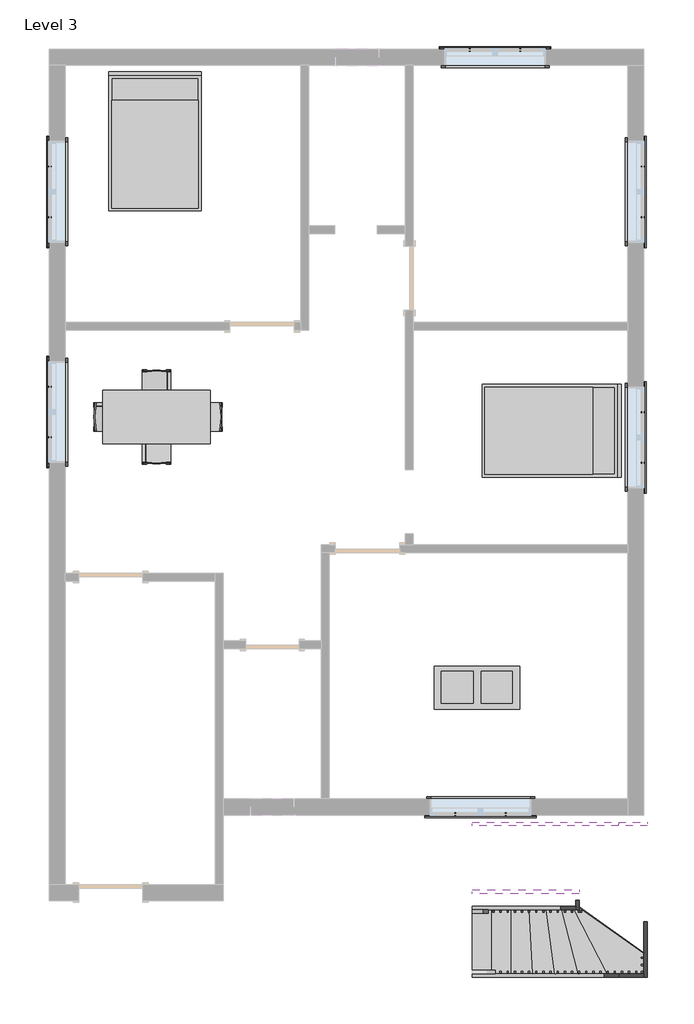
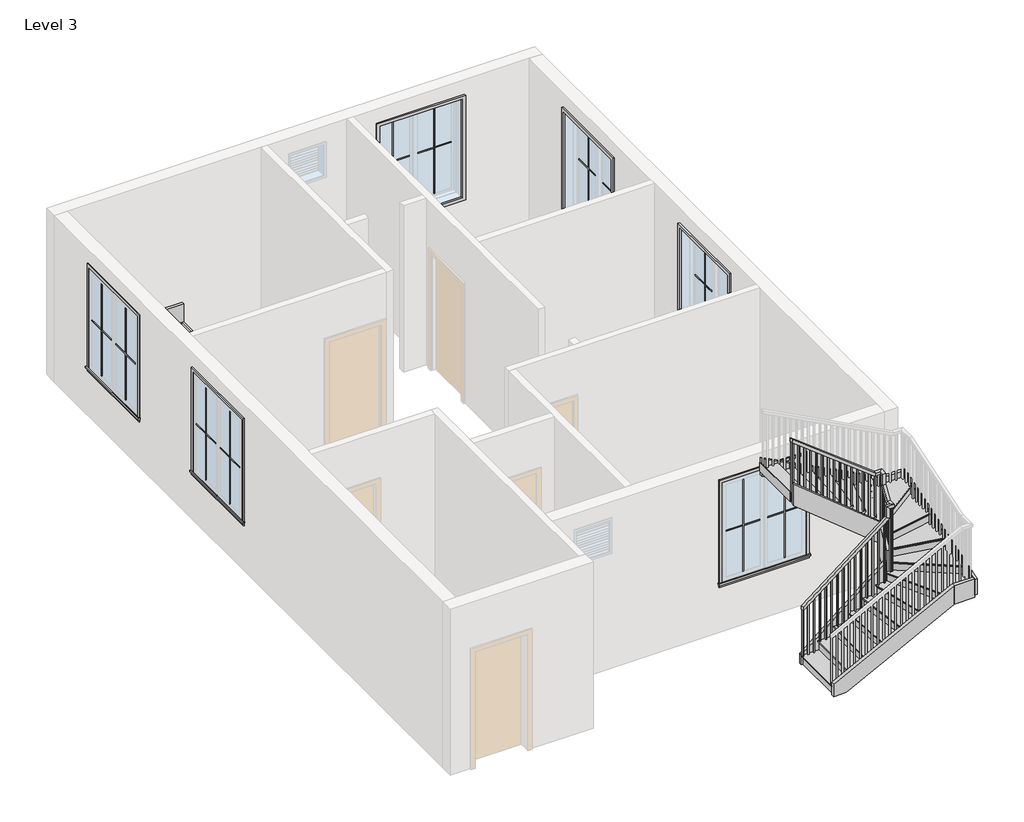
# One storey, part 3 of 3: 25 proxies, 8 members, 3 furniture elements, 1 railing, 1 stair flight.
"""IFC4 building model written with IfcOpenShell, lengths in millimetres."""

from ifc_helpers import new_model, si_unit, frame, origin, place, context, project, spatial, polyline, outline, extrude, faceted_brep, transform, mapped, element, save
from components import muntin_pattern_2x2_muntin_pattern_2x2_bff912c5, muntin_pattern_2x2_muntin_pattern_2x2_c2194282, trim_window_exterior_flat_with_sill_e04b3088, trim_window_interior_flat_picture_frame_2a7685fe, coffee_table_with_brass_mullions_11320_coffee_table_with_5962bef7, bed_17739_bed_17739_15c61121, dining_table_w_chairs_11374_0cdfc61b, stair_flight_4f848c3a

model = new_model("IFC4")

# Units and contexts
model_context = context("Model", 3, world=origin())
ifc_project = project(units=[si_unit("LENGTHUNIT", "METRE", prefix="MILLI")], contexts=[model_context])

# Site, building, storey
site = spatial("IfcSite", under=ifc_project)
building = spatial("IfcBuilding", under=site)
storey = spatial("IfcBuildingStorey", under=building, Name="Level 3", Elevation=3200.4)

# Proxies
placement = place(None, origin())
muntin_pattern_2x2_muntin_pattern_2x2_shape = muntin_pattern_2x2_muntin_pattern_2x2_bff912c5(model_context)
element("IfcBuildingElementProxy", 1, Name="Muntin Pattern_2x2 : Muntin Pattern_2x2", ObjectType="Muntin Pattern_2x2 : Muntin Pattern_2x2", at=placement, inside=storey, context=model_context, shape_type="MappedRepresentation", body=[
    mapped(muntin_pattern_2x2_muntin_pattern_2x2_shape, transform((2964.3605034, 427.8534591, 4184.65), x_axis=(0.0, -1.0, 0.0), y_axis=(1.0, 0.0, 0.0), z_axis=(0.0, 0.0, 1.0))),
])
element("IfcBuildingElementProxy", 2, Name="Muntin Pattern_2x2 : Muntin Pattern_2x2", ObjectType="Muntin Pattern_2x2 : Muntin Pattern_2x2", at=placement, inside=storey, context=model_context, shape_type="MappedRepresentation", body=[
    mapped(muntin_pattern_2x2_muntin_pattern_2x2_shape, transform((2964.3605034, 3923.5284591, 4184.65), x_axis=(0.0, -1.0, 0.0), y_axis=(1.0, 0.0, 0.0), z_axis=(0.0, 0.0, 1.0))),
])
element("IfcBuildingElementProxy", 3, Name="Muntin Pattern_2x2 : Muntin Pattern_2x2", ObjectType="Muntin Pattern_2x2 : Muntin Pattern_2x2", at=placement, inside=storey, context=model_context, shape_type="MappedRepresentation", body=[
    mapped(muntin_pattern_2x2_muntin_pattern_2x2_shape, transform((498.9730034, 5582.4659591, 4184.65), x_axis=(1.0, 0.0, 0.0), y_axis=(0.0, 1.0, 0.0), z_axis=(0.0, 0.0, 1.0))),
])
element("IfcBuildingElementProxy", 4, Name="Muntin Pattern_2x2 : Muntin Pattern_2x2", ObjectType="Muntin Pattern_2x2 : Muntin Pattern_2x2", at=placement, inside=storey, context=model_context, shape_type="MappedRepresentation", body=[
    mapped(muntin_pattern_2x2_muntin_pattern_2x2_shape, transform((-5474.7894966, 3202.8034591, 4184.65), x_axis=(0.0, 1.0, 0.0), y_axis=(-1.0, 0.0, 0.0), z_axis=(0.0, 0.0, 1.0))),
])
element("IfcBuildingElementProxy", 5, Name="Muntin Pattern_2x2 : Muntin Pattern_2x2", ObjectType="Muntin Pattern_2x2 : Muntin Pattern_2x2", at=placement, inside=storey, context=model_context, shape_type="MappedRepresentation", body=[
    mapped(muntin_pattern_2x2_muntin_pattern_2x2_shape, transform((-5474.7894966, 69.0784591, 4184.65), x_axis=(0.0, 1.0, 0.0), y_axis=(-1.0, 0.0, 0.0), z_axis=(0.0, 0.0, 1.0))),
])
element("IfcBuildingElementProxy", 6, Name="Muntin Pattern_2x2 : Muntin Pattern_2x2", ObjectType="Muntin Pattern_2x2 : Muntin Pattern_2x2", at=placement, inside=storey, context=model_context, shape_type="MappedRepresentation", body=[
    mapped(muntin_pattern_2x2_muntin_pattern_2x2_shape, transform((1013.3230034, -5295.0840409, 4184.65), x_axis=(-1.0, 0.0, 0.0), y_axis=(0.0, -1.0, 0.0), z_axis=(0.0, 0.0, 1.0))),
])
muntin_pattern_2x2_muntin_pattern_2x2_2_shape = muntin_pattern_2x2_muntin_pattern_2x2_c2194282(model_context)
element("IfcBuildingElementProxy", 7, Name="Muntin Pattern_2x2 : Muntin Pattern_2x2", ObjectType="Muntin Pattern_2x2 : Muntin Pattern_2x2", at=placement, inside=storey, context=model_context, shape_type="MappedRepresentation", body=[
    mapped(muntin_pattern_2x2_muntin_pattern_2x2_2_shape, transform((2964.3605034, -292.8715409, 4184.65), x_axis=(0.0, 1.0, 0.0), y_axis=(-1.0, 0.0, 0.0), z_axis=(0.0, 0.0, 1.0))),
])
element("IfcBuildingElementProxy", 8, Name="Muntin Pattern_2x2 : Muntin Pattern_2x2", ObjectType="Muntin Pattern_2x2 : Muntin Pattern_2x2", at=placement, inside=storey, context=model_context, shape_type="MappedRepresentation", body=[
    mapped(muntin_pattern_2x2_muntin_pattern_2x2_2_shape, transform((2964.3605034, 3202.8034591, 4184.65), x_axis=(0.0, 1.0, 0.0), y_axis=(-1.0, 0.0, 0.0), z_axis=(0.0, 0.0, 1.0))),
])
element("IfcBuildingElementProxy", 9, Name="Muntin Pattern_2x2 : Muntin Pattern_2x2", ObjectType="Muntin Pattern_2x2 : Muntin Pattern_2x2", at=placement, inside=storey, context=model_context, shape_type="MappedRepresentation", body=[
    mapped(muntin_pattern_2x2_muntin_pattern_2x2_2_shape, transform((1219.6980034, 5582.4659591, 4184.65), x_axis=(-1.0, 0.0, 0.0), y_axis=(0.0, -1.0, 0.0), z_axis=(0.0, 0.0, 1.0))),
])
element("IfcBuildingElementProxy", 10, Name="Muntin Pattern_2x2 : Muntin Pattern_2x2", ObjectType="Muntin Pattern_2x2 : Muntin Pattern_2x2", at=placement, inside=storey, context=model_context, shape_type="MappedRepresentation", body=[
    mapped(muntin_pattern_2x2_muntin_pattern_2x2_2_shape, transform((-5474.7894966, 3923.5284591, 4184.65), x_axis=(0.0, -1.0, 0.0), y_axis=(1.0, 0.0, 0.0), z_axis=(0.0, 0.0, 1.0))),
])
element("IfcBuildingElementProxy", 11, Name="Muntin Pattern_2x2 : Muntin Pattern_2x2", ObjectType="Muntin Pattern_2x2 : Muntin Pattern_2x2", at=placement, inside=storey, context=model_context, shape_type="MappedRepresentation", body=[
    mapped(muntin_pattern_2x2_muntin_pattern_2x2_2_shape, transform((-5474.7894966, 789.8034591, 4184.65), x_axis=(0.0, -1.0, 0.0), y_axis=(1.0, 0.0, 0.0), z_axis=(0.0, 0.0, 1.0))),
])
element("IfcBuildingElementProxy", 12, Name="Muntin Pattern_2x2 : Muntin Pattern_2x2", ObjectType="Muntin Pattern_2x2 : Muntin Pattern_2x2", at=placement, inside=storey, context=model_context, shape_type="MappedRepresentation", body=[
    mapped(muntin_pattern_2x2_muntin_pattern_2x2_2_shape, transform((292.5980034, -5295.0840409, 4184.65), x_axis=(1.0, 0.0, 0.0), y_axis=(0.0, 1.0, 0.0), z_axis=(0.0, 0.0, 1.0))),
])
trim_window_exterior_flat_with_sill_shape = trim_window_exterior_flat_with_sill_e04b3088(model_context)
element("IfcBuildingElementProxy", 13, Name="Trim-Window-Exterior-Flat : with Sill", ObjectType="Trim-Window-Exterior-Flat : with Sill", at=placement, inside=storey, context=model_context, shape_type="MappedRepresentation", body=[
    mapped(trim_window_exterior_flat_with_sill_shape, transform((2973.8855034, 67.4909591, 5943.6), x_axis=(0.0, 1.0, 0.0), y_axis=(0.0, 0.0, 1.0), z_axis=(1.0, 0.0, 0.0))),
])
element("IfcBuildingElementProxy", 14, Name="Trim-Window-Exterior-Flat : with Sill", ObjectType="Trim-Window-Exterior-Flat : with Sill", at=placement, inside=storey, context=model_context, shape_type="MappedRepresentation", body=[
    mapped(trim_window_exterior_flat_with_sill_shape, transform((2973.8855034, 3563.1659591, 5943.6), x_axis=(0.0, 1.0, 0.0), y_axis=(0.0, 0.0, 1.0), z_axis=(1.0, 0.0, 0.0))),
])
element("IfcBuildingElementProxy", 15, Name="Trim-Window-Exterior-Flat : with Sill", ObjectType="Trim-Window-Exterior-Flat : with Sill", at=placement, inside=storey, context=model_context, shape_type="MappedRepresentation", body=[
    mapped(trim_window_exterior_flat_with_sill_shape, transform((859.3355034, 5591.9909591, 5943.6), x_axis=(-1.0, 0.0, 0.0), y_axis=(0.0, 0.0, 1.0), z_axis=(0.0, 1.0, 0.0))),
])
element("IfcBuildingElementProxy", 16, Name="Trim-Window-Exterior-Flat : with Sill", ObjectType="Trim-Window-Exterior-Flat : with Sill", at=placement, inside=storey, context=model_context, shape_type="MappedRepresentation", body=[
    mapped(trim_window_exterior_flat_with_sill_shape, transform((-5484.3144966, 3563.1659591, 5943.6), x_axis=(0.0, -1.0, 0.0), y_axis=(0.0, 0.0, 1.0), z_axis=(-1.0, 0.0, 0.0))),
])
element("IfcBuildingElementProxy", 17, Name="Trim-Window-Exterior-Flat : with Sill", ObjectType="Trim-Window-Exterior-Flat : with Sill", at=placement, inside=storey, context=model_context, shape_type="MappedRepresentation", body=[
    mapped(trim_window_exterior_flat_with_sill_shape, transform((-5484.3144966, 429.4409591, 5943.6), x_axis=(0.0, -1.0, 0.0), y_axis=(0.0, 0.0, 1.0), z_axis=(-1.0, 0.0, 0.0))),
])
element("IfcBuildingElementProxy", 18, Name="Trim-Window-Exterior-Flat : with Sill", ObjectType="Trim-Window-Exterior-Flat : with Sill", at=placement, inside=storey, context=model_context, shape_type="MappedRepresentation", body=[
    mapped(trim_window_exterior_flat_with_sill_shape, transform((652.9605034, -5304.6090409, 5943.6), x_axis=(1.0, 0.0, 0.0), y_axis=(0.0, 0.0, 1.0), z_axis=(0.0, -1.0, 0.0))),
])
trim_window_interior_flat_picture_frame_shape = trim_window_interior_flat_picture_frame_2a7685fe(model_context)
element("IfcBuildingElementProxy", 19, Name="Trim-Window-Interior-Flat : Picture Frame", ObjectType="Trim-Window-Interior-Flat : Picture Frame", at=placement, inside=storey, context=model_context, shape_type="MappedRepresentation", body=[
    mapped(trim_window_interior_flat_picture_frame_shape, transform((2745.2855034, 67.4909591, 5943.6), x_axis=(0.0, -1.0, 0.0), y_axis=(0.0, 0.0, 1.0), z_axis=(-1.0, 0.0, 0.0))),
])
element("IfcBuildingElementProxy", 20, Name="Trim-Window-Interior-Flat : Picture Frame", ObjectType="Trim-Window-Interior-Flat : Picture Frame", at=placement, inside=storey, context=model_context, shape_type="MappedRepresentation", body=[
    mapped(trim_window_interior_flat_picture_frame_shape, transform((2745.2855034, 3563.1659591, 5943.6), x_axis=(0.0, -1.0, 0.0), y_axis=(0.0, 0.0, 1.0), z_axis=(-1.0, 0.0, 0.0))),
])
element("IfcBuildingElementProxy", 21, Name="Trim-Window-Interior-Flat : Picture Frame", ObjectType="Trim-Window-Interior-Flat : Picture Frame", at=placement, inside=storey, context=model_context, shape_type="MappedRepresentation", body=[
    mapped(trim_window_interior_flat_picture_frame_shape, transform((859.3355034, 5363.3909591, 5943.6), x_axis=(1.0, 0.0, 0.0), y_axis=(0.0, 0.0, 1.0), z_axis=(0.0, -1.0, 0.0))),
])
element("IfcBuildingElementProxy", 22, Name="Trim-Window-Interior-Flat : Picture Frame", ObjectType="Trim-Window-Interior-Flat : Picture Frame", at=placement, inside=storey, context=model_context, shape_type="MappedRepresentation", body=[
    mapped(trim_window_interior_flat_picture_frame_shape, transform((-5255.7144966, 3563.1659591, 5943.6), x_axis=(0.0, 1.0, 0.0), y_axis=(0.0, 0.0, 1.0), z_axis=(1.0, 0.0, 0.0))),
])
element("IfcBuildingElementProxy", 23, Name="Trim-Window-Interior-Flat : Picture Frame", ObjectType="Trim-Window-Interior-Flat : Picture Frame", at=placement, inside=storey, context=model_context, shape_type="MappedRepresentation", body=[
    mapped(trim_window_interior_flat_picture_frame_shape, transform((-5255.7144966, 429.4409591, 5943.6), x_axis=(0.0, 1.0, 0.0), y_axis=(0.0, 0.0, 1.0), z_axis=(1.0, 0.0, 0.0))),
])
element("IfcBuildingElementProxy", 24, Name="Trim-Window-Interior-Flat : Picture Frame", ObjectType="Trim-Window-Interior-Flat : Picture Frame", at=placement, inside=storey, context=model_context, shape_type="MappedRepresentation", body=[
    mapped(trim_window_interior_flat_picture_frame_shape, transform((652.9605034, -5076.0090409, 5943.6), x_axis=(-1.0, 0.0, 0.0), y_axis=(0.0, 0.0, 1.0), z_axis=(0.0, 1.0, 0.0))),
])
coffee_table_with_brass_mullions_11320_coffee_table_with_shape = coffee_table_with_brass_mullions_11320_coffee_table_with_5962bef7(model_context)
element("IfcBuildingElementProxy", 25, Name="coffee_table_with_brass_mullions_11320 : coffee_table_with_brass_mullions_11320", ObjectType="coffee_table_with_brass_mullions_11320 : coffee_table_with_brass_mullions_11320", at=placement, inside=storey, context=model_context, shape_type="MappedRepresentation", body=[
    mapped(coffee_table_with_brass_mullions_11320_coffee_table_with_shape, transform((1240.0943553, -3926.0808329, 3200.4), x_axis=(1.0, 0.0, 0.0), y_axis=(0.0, 1.0, 0.0), z_axis=(0.0, 0.0, 1.0))),
])

# Furniture
bed_17739_bed_17739_shape = bed_17739_bed_17739_15c61121(model_context)
element("IfcFurniture", 26, ObjectType="Bed_17739 : Bed_17739", at=placement, inside=storey, context=model_context, shape_type="MappedRepresentation", body=[
    mapped(bed_17739_bed_17739_shape, transform((-3979.3644966, 4258.4909591, 3200.4), x_axis=(1.0, 0.0, 0.0), y_axis=(0.0, 1.0, 0.0), z_axis=(0.0, 0.0, 1.0))),
])
element("IfcFurniture", 27, ObjectType="Bed_17739 : Bed_17739", at=placement, inside=storey, context=model_context, shape_type="MappedRepresentation", body=[
    mapped(bed_17739_bed_17739_shape, transform((1640.3855034, 162.7409591, 3200.4), x_axis=(0.0, -1.0, 0.0), y_axis=(1.0, 0.0, 0.0), z_axis=(0.0, 0.0, 1.0))),
])
dining_table_w_chairs_11374_shape = dining_table_w_chairs_11374_0cdfc61b(model_context)
element("IfcFurniture", 28, ObjectType="Dining_Table_w_Chairs_11374", at=placement, inside=storey, context=model_context, shape_type="MappedRepresentation", body=[
    mapped(dining_table_w_chairs_11374_shape, transform((-3975.2132663, 265.1952874, 3200.4), x_axis=(1.0, 0.0, 0.0), y_axis=(0.0, 1.0, 0.0), z_axis=(0.0, 0.0, 1.0))),
])

# Members
element("IfcMember", 29, ObjectType="Stringer - 2\" Width", at=placement, inside=storey, context=model_context, shape_type="SweptSolid", body=[
    extrude(outline(polyline([(3376.5764461, 531.7538115), (3200.4, 531.7538115), (3200.4, 798.0154561), (4187.5410923, 2008.6855034), (4580.818648, 2008.6855034), (3376.5764461, 531.7538115)])), frame((0.0, -6650.8090409, 0.0), z_axis=(0.0, 1.0, 0.0), x_axis=(0.0, 0.0, 1.0)), (0.0, 0.0, 1.0), 50.8),
])
element("IfcMember", 30, ObjectType="Stringer - 2\" Width", at=placement, inside=storey, context=model_context, shape_type="SweptSolid", body=[
    extrude(outline(polyline([(-6650.8090409, 4228.9617647), (-6650.8090409, 4773.6682978), (-6444.1719234, 5126.5409689), (-6422.2090409, 5126.5409689), (-6422.2090409, 4560.865107), (-6616.5668235, 4228.9617647), (-6650.8090409, 4228.9617647)])), frame((2008.6855034, 0.0, 0.0), z_axis=(1.0, 0.0, 0.0), x_axis=(0.0, 1.0, 0.0)), (0.0, 0.0, 1.0), 50.8),
])
element("IfcMember", 31, ObjectType="Stringer - 2\" Width", at=placement, inside=storey, context=model_context, shape_type="SweptSolid", body=[
    extrude(outline(polyline([(4733.2634131, 2059.4855034), (5126.5409689, 2059.4855034), (6372.2038432, 531.7538115), (5978.9262875, 531.7538115), (4733.2634131, 2059.4855034)])), frame((0.0, -6422.2090409, 0.0), z_axis=(0.0, 1.0, 0.0), x_axis=(0.0, 0.0, 1.0)), (0.0, 0.0, 1.0), 50.8),
])
element("IfcMember", 32, ObjectType="Stringer - 2\" Width", at=placement, inside=storey, context=model_context, shape_type="SweptSolid", body=[
    extrude(outline(polyline([(3430.039954, 531.7538115), (3200.4, 531.7538115), (3200.4, 751.5161291), (4162.900629, 2619.1710032), (4505.7956453, 2619.1710032), (3430.039954, 531.7538115)])), frame((0.0, -7616.0090409, 0.0), z_axis=(0.0, 1.0, 0.0), x_axis=(0.0, 0.0, 1.0)), (0.0, 0.0, 1.0), 50.8),
])
element("IfcMember", 33, ObjectType="Stringer - 2\" Width", at=placement, inside=storey, context=model_context, shape_type="SweptSolid", body=[
    extrude(outline(polyline([(2619.1710032, -7616.0090409), (2619.1710032, -7565.2090409), (2973.8855034, -7565.2090409), (2973.8855034, -7616.0090409), (2619.1710032, -7616.0090409)])), frame((0.0, 0.0, 4162.900629), z_axis=(0.0, 0.0, 1.0), x_axis=(1.0, 0.0, 0.0)), (0.0, 0.0, 1.0), 342.8950162),
])
element("IfcMember", 34, ObjectType="Stringer - 2\" Width", at=placement, inside=storey, context=model_context, shape_type="SweptSolid", body=[
    extrude(outline(polyline([(-7616.0090409, 4200.9956453), (-7616.0090409, 4489.4952212), (-5493.9891581, 5170.3972697), (-5457.0090409, 5170.3972697), (-5457.0090409, 4839.3682298), (-7446.4865579, 4200.9956453), (-7616.0090409, 4200.9956453)])), frame((2973.8855034, 0.0, 0.0), z_axis=(1.0, 0.0, 0.0), x_axis=(0.0, 1.0, 0.0)), (0.0, 0.0, 1.0), 50.8),
])
element("IfcMember", 35, ObjectType="Stringer - 2\" Width", at=placement, inside=storey, context=model_context, shape_type="SweptSolid", body=[
    extrude(outline(polyline([(3024.6855034, -5406.2090409), (3024.6855034, -5457.0090409), (2619.1710032, -5457.0090409), (2619.1710032, -5406.2090409), (3024.6855034, -5406.2090409)])), frame((0.0, 0.0, 4850.2904473), z_axis=(0.0, 0.0, 1.0), x_axis=(1.0, 0.0, 0.0)), (0.0, 0.0, 1.0), 320.1068224),
])
element("IfcMember", 36, ObjectType="Stringer - 2\" Width", at=placement, inside=storey, context=model_context, shape_type="SweptSolid", body=[
    extrude(outline(polyline([(4850.2904473, 2619.1710032), (5170.3972697, 2619.1710032), (6246.1529609, 531.7538115), (5926.0461385, 531.7538115), (4850.2904473, 2619.1710032)])), frame((0.0, -5457.0090409, 0.0), z_axis=(0.0, 1.0, 0.0), x_axis=(0.0, 0.0, 1.0)), (0.0, 0.0, 1.0), 50.8),
])

# Railing
element("IfcRailing", 37, ObjectType="Handrail - Rectangular", at=placement, inside=storey, context=model_context, shape_type="SolidModel", body=[
    faceted_brep([(531.7538115, -6650.8090409, 4284.1333333), (531.7538115, -6650.8090409, 4219.8000346), (531.7538115, -6701.6090409, 4219.8000346), (531.7538115, -6701.6090409, 4284.1333333), (1983.2855034, -6650.8090409, 5412.0191036), (2034.0855034, -6650.8090409, 5387.1590024), (2034.0855034, -6701.6090409, 5387.1590024), (1983.2855034, -6701.6090409, 5412.0191036), (2059.4855034, -6545.487707, 5564.2281882), (2059.4855034, -6574.6090409, 5615.0281882), (2059.4855034, -6447.6090409, 5831.9051451), (2059.4855034, -6396.8090409, 5818.1256424), (2110.2855034, -6545.487707, 5564.2281882), (2110.2855034, -6396.8090409, 5818.1256424), (2110.2855034, -6574.6090409, 5615.0281882), (2110.2855034, -6447.6090409, 5831.9051451), (531.7538115, -6371.4090409, 7162.8), (531.7538115, -6320.6090409, 7162.8), (531.7538115, -6320.6090409, 7098.4667013), (531.7538115, -6371.4090409, 7098.4667013), (1965.8688354, -6371.4090409, 5984.1142297), (1983.2855034, -6371.4090409, 6034.9142297), (1965.8688354, -6320.6090409, 5984.1142297), (1983.2855034, -6320.6090409, 6034.9142297), (1983.2855034, -6650.8090409, 5615.0281882), (2034.0855034, -6650.8090409, 5564.2281882), (2034.0855034, -6701.6090409, 5564.2281882), (1983.2855034, -6701.6090409, 5615.0281882), (2059.4855034, -6650.8090409, 5615.0281882), (2059.4855034, -6650.8090409, 5564.2281882), (2110.2855034, -6701.6090409, 5564.2281882), (2110.2855034, -6701.6090409, 5615.0281882), (2059.4855034, -6447.6090409, 6034.9142297), (2059.4855034, -6396.8090409, 5984.1142297), (2110.2855034, -6396.8090409, 5984.1142297), (2110.2855034, -6447.6090409, 6034.9142297), (2059.4855034, -6371.4090409, 6034.9142297), (2059.4855034, -6371.4090409, 5984.1142297), (2110.2855034, -6320.6090409, 5984.1142297), (2110.2855034, -6320.6090409, 6034.9142297)], [[[0, 1, 2, 3]], [[1, 0, 4, 5]], [[2, 1, 5, 6]], [[3, 2, 6, 7]], [[0, 3, 7, 4]], [[8, 9, 10, 11]], [[12, 8, 11, 13]], [[14, 12, 13, 15]], [[9, 14, 15, 10]], [[16, 17, 18, 19]], [[20, 21, 16, 19]], [[22, 20, 19, 18]], [[23, 22, 18, 17]], [[21, 23, 17, 16]], [[5, 4, 24, 25]], [[6, 5, 25, 26]], [[7, 6, 26, 27]], [[4, 7, 27, 24]], [[25, 24, 28, 29]], [[26, 25, 29, 30]], [[27, 26, 30, 31]], [[24, 27, 31, 28]], [[29, 28, 9, 8]], [[30, 29, 8, 12]], [[31, 30, 12, 14]], [[28, 31, 14, 9]], [[11, 10, 32, 33]], [[13, 11, 33, 34]], [[15, 13, 34, 35]], [[10, 15, 35, 32]], [[33, 32, 36, 37]], [[34, 33, 37, 38]], [[35, 34, 38, 39]], [[32, 35, 39, 36]], [[37, 36, 21, 20]], [[38, 37, 20, 22]], [[39, 38, 22, 23]], [[36, 39, 23, 21]]]),
    extrude(outline(polyline([(7083.2316852, 551.3605034), (6079.0666667, 551.3605034), (6079.0666667, 570.4105034), (7068.4292361, 570.4105034), (7083.2316852, 551.3605034)])), frame((0.0, -6355.5340409, 0.0), z_axis=(0.0, 1.0, 0.0), x_axis=(0.0, 0.0, 1.0)), (0.0, 0.0, 1.0), 19.05),
    extrude(outline(polyline([(7004.2852902, 652.9605034), (6079.0666667, 652.9605034), (6079.0666667, 672.0105034), (6989.4828411, 672.0105034), (7004.2852902, 652.9605034)])), frame((0.0, -6355.5340409, 0.0), z_axis=(0.0, 1.0, 0.0), x_axis=(0.0, 0.0, 1.0)), (0.0, 0.0, 1.0), 19.05),
    extrude(outline(polyline([(6925.3388952, 754.5605034), (6079.0666667, 754.5605034), (6079.0666667, 773.6105034), (6910.5364462, 773.6105034), (6925.3388952, 754.5605034)])), frame((0.0, -6355.5340409, 0.0), z_axis=(0.0, 1.0, 0.0), x_axis=(0.0, 0.0, 1.0)), (0.0, 0.0, 1.0), 19.05),
    extrude(outline(polyline([(6846.3925003, 856.1605034), (5909.7333333, 856.1605034), (5909.7333333, 875.2105034), (6831.5900512, 875.2105034), (6846.3925003, 856.1605034)])), frame((0.0, -6355.5340409, 0.0), z_axis=(0.0, 1.0, 0.0), x_axis=(0.0, 0.0, 1.0)), (0.0, 0.0, 1.0), 19.05),
    extrude(outline(polyline([(6767.4461053, 957.7605034), (5909.7333333, 957.7605034), (5909.7333333, 976.8105034), (6752.6436562, 976.8105034), (6767.4461053, 957.7605034)])), frame((0.0, -6355.5340409, 0.0), z_axis=(0.0, 1.0, 0.0), x_axis=(0.0, 0.0, 1.0)), (0.0, 0.0, 1.0), 19.05),
    extrude(outline(polyline([(6688.4997103, 1059.3605034), (5909.7333333, 1059.3605034), (5909.7333333, 1078.4105034), (6673.6972613, 1078.4105034), (6688.4997103, 1059.3605034)])), frame((0.0, -6355.5340409, 0.0), z_axis=(0.0, 1.0, 0.0), x_axis=(0.0, 0.0, 1.0)), (0.0, 0.0, 1.0), 19.05),
    extrude(outline(polyline([(6609.5533154, 1160.9605034), (5740.4, 1160.9605034), (5740.4, 1180.0105034), (6594.7508663, 1180.0105034), (6609.5533154, 1160.9605034)])), frame((0.0, -6355.5340409, 0.0), z_axis=(0.0, 1.0, 0.0), x_axis=(0.0, 0.0, 1.0)), (0.0, 0.0, 1.0), 19.05),
    extrude(outline(polyline([(6530.6069204, 1262.5605034), (5740.4, 1262.5605034), (5740.4, 1281.6105034), (6515.8044713, 1281.6105034), (6530.6069204, 1262.5605034)])), frame((0.0, -6355.5340409, 0.0), z_axis=(0.0, 1.0, 0.0), x_axis=(0.0, 0.0, 1.0)), (0.0, 0.0, 1.0), 19.05),
    extrude(outline(polyline([(6451.6605254, 1364.1605034), (5571.0666667, 1364.1605034), (5571.0666667, 1383.2105034), (6436.8580764, 1383.2105034), (6451.6605254, 1364.1605034)])), frame((0.0, -6355.5340409, 0.0), z_axis=(0.0, 1.0, 0.0), x_axis=(0.0, 0.0, 1.0)), (0.0, 0.0, 1.0), 19.05),
    extrude(outline(polyline([(6372.7141304, 1465.7605034), (5571.0666667, 1465.7605034), (5571.0666667, 1484.8105034), (6357.9116814, 1484.8105034), (6372.7141304, 1465.7605034)])), frame((0.0, -6355.5340409, 0.0), z_axis=(0.0, 1.0, 0.0), x_axis=(0.0, 0.0, 1.0)), (0.0, 0.0, 1.0), 19.05),
    extrude(outline(polyline([(6293.7677355, 1567.3605034), (5571.0666667, 1567.3605034), (5571.0666667, 1586.4105034), (6278.9652864, 1586.4105034), (6293.7677355, 1567.3605034)])), frame((0.0, -6355.5340409, 0.0), z_axis=(0.0, 1.0, 0.0), x_axis=(0.0, 0.0, 1.0)), (0.0, 0.0, 1.0), 19.05),
    extrude(outline(polyline([(6214.8213405, 1668.9605034), (5401.7333333, 1668.9605034), (5401.7333333, 1688.0105034), (6200.0188914, 1688.0105034), (6214.8213405, 1668.9605034)])), frame((0.0, -6355.5340409, 0.0), z_axis=(0.0, 1.0, 0.0), x_axis=(0.0, 0.0, 1.0)), (0.0, 0.0, 1.0), 19.05),
    extrude(outline(polyline([(6135.8749455, 1770.5605034), (5401.7333333, 1770.5605034), (5401.7333333, 1789.6105034), (6121.0724965, 1789.6105034), (6135.8749455, 1770.5605034)])), frame((0.0, -6355.5340409, 0.0), z_axis=(0.0, 1.0, 0.0), x_axis=(0.0, 0.0, 1.0)), (0.0, 0.0, 1.0), 19.05),
    extrude(outline(polyline([(6056.9285506, 1872.1605034), (5232.4, 1872.1605034), (5232.4, 1891.2105034), (6042.1261015, 1891.2105034), (6056.9285506, 1872.1605034)])), frame((0.0, -6355.5340409, 0.0), z_axis=(0.0, 1.0, 0.0), x_axis=(0.0, 0.0, 1.0)), (0.0, 0.0, 1.0), 19.05),
    extrude(outline(polyline([(5977.9821556, 1973.7605034), (5232.4, 1973.7605034), (5232.4, 1992.8105034), (5963.1797065, 1992.8105034), (5977.9821556, 1973.7605034)])), frame((0.0, -6355.5340409, 0.0), z_axis=(0.0, 1.0, 0.0), x_axis=(0.0, 0.0, 1.0)), (0.0, 0.0, 1.0), 19.05),
    extrude(outline(polyline([(2075.3605034, -6380.9340409), (2075.3605034, -6361.8840409), (2094.4105034, -6361.8840409), (2094.4105034, -6380.9340409), (2075.3605034, -6380.9340409)])), frame((0.0, 0.0, 4893.7333333), z_axis=(0.0, 0.0, 1.0), x_axis=(1.0, 0.0, 0.0)), (0.0, 0.0, 1.0), 1090.3808964),
    extrude(outline(polyline([(-6463.4840409, 5704.26524), (-6463.4840409, 4724.4), (-6482.5340409, 4724.4), (-6482.5340409, 5671.7336964), (-6463.4840409, 5704.26524)])), frame((2075.3605034, 0.0, 0.0), z_axis=(1.0, 0.0, 0.0), x_axis=(0.0, 1.0, 0.0)), (0.0, 0.0, 1.0), 19.05),
    extrude(outline(polyline([(-6565.0840409, 5530.7636744), (-6565.0840409, 4555.0666667), (-6584.1340409, 4555.0666667), (-6584.1340409, 5498.2321309), (-6565.0840409, 5530.7636744)])), frame((2075.3605034, 0.0, 0.0), z_axis=(1.0, 0.0, 0.0), x_axis=(0.0, 1.0, 0.0)), (0.0, 0.0, 1.0), 19.05),
    extrude(outline(polyline([(2046.2288115, -6666.6840409), (2065.2788115, -6666.6840409), (2065.2788115, -6685.7340409), (2046.2288115, -6685.7340409), (2046.2288115, -6666.6840409)])), frame((0.0, 0.0, 4385.7333333), z_axis=(0.0, 0.0, 1.0), x_axis=(1.0, 0.0, 0.0)), (0.0, 0.0, 1.0), 1178.4948549),
    extrude(outline(polyline([(5317.6483397, 1944.6288115), (4216.4, 1944.6288115), (4216.4, 1963.6788115), (5332.4507888, 1963.6788115), (5317.6483397, 1944.6288115)])), frame((0.0, -6685.7340409, 0.0), z_axis=(0.0, 1.0, 0.0), x_axis=(0.0, 0.0, 1.0)), (0.0, 0.0, 1.0), 19.05),
    extrude(outline(polyline([(5238.7019447, 1843.0288115), (4216.4, 1843.0288115), (4216.4, 1862.0788115), (5253.5043938, 1862.0788115), (5238.7019447, 1843.0288115)])), frame((0.0, -6685.7340409, 0.0), z_axis=(0.0, 1.0, 0.0), x_axis=(0.0, 0.0, 1.0)), (0.0, 0.0, 1.0), 19.05),
    extrude(outline(polyline([(5159.7555498, 1741.4288115), (4047.0666667, 1741.4288115), (4047.0666667, 1760.4788115), (5174.5579988, 1760.4788115), (5159.7555498, 1741.4288115)])), frame((0.0, -6685.7340409, 0.0), z_axis=(0.0, 1.0, 0.0), x_axis=(0.0, 0.0, 1.0)), (0.0, 0.0, 1.0), 19.05),
    extrude(outline(polyline([(5080.8091548, 1639.8288115), (4047.0666667, 1639.8288115), (4047.0666667, 1658.8788115), (5095.6116039, 1658.8788115), (5080.8091548, 1639.8288115)])), frame((0.0, -6685.7340409, 0.0), z_axis=(0.0, 1.0, 0.0), x_axis=(0.0, 0.0, 1.0)), (0.0, 0.0, 1.0), 19.05),
    extrude(outline(polyline([(5001.8627598, 1538.2288115), (3877.7333333, 1538.2288115), (3877.7333333, 1557.2788115), (5016.6652089, 1557.2788115), (5001.8627598, 1538.2288115)])), frame((0.0, -6685.7340409, 0.0), z_axis=(0.0, 1.0, 0.0), x_axis=(0.0, 0.0, 1.0)), (0.0, 0.0, 1.0), 19.05),
    extrude(outline(polyline([(4922.9163649, 1436.6288115), (3877.7333333, 1436.6288115), (3877.7333333, 1455.6788115), (4937.7188139, 1455.6788115), (4922.9163649, 1436.6288115)])), frame((0.0, -6685.7340409, 0.0), z_axis=(0.0, 1.0, 0.0), x_axis=(0.0, 0.0, 1.0)), (0.0, 0.0, 1.0), 19.05),
    extrude(outline(polyline([(4843.9699699, 1335.0288115), (3708.4, 1335.0288115), (3708.4, 1354.0788115), (4858.7724189, 1354.0788115), (4843.9699699, 1335.0288115)])), frame((0.0, -6685.7340409, 0.0), z_axis=(0.0, 1.0, 0.0), x_axis=(0.0, 0.0, 1.0)), (0.0, 0.0, 1.0), 19.05),
    extrude(outline(polyline([(4765.0235749, 1233.4288115), (3708.4, 1233.4288115), (3708.4, 1252.4788115), (4779.826024, 1252.4788115), (4765.0235749, 1233.4288115)])), frame((0.0, -6685.7340409, 0.0), z_axis=(0.0, 1.0, 0.0), x_axis=(0.0, 0.0, 1.0)), (0.0, 0.0, 1.0), 19.05),
    extrude(outline(polyline([(4686.0771799, 1131.8288115), (3708.4, 1131.8288115), (3708.4, 1150.8788115), (4700.879629, 1150.8788115), (4686.0771799, 1131.8288115)])), frame((0.0, -6685.7340409, 0.0), z_axis=(0.0, 1.0, 0.0), x_axis=(0.0, 0.0, 1.0)), (0.0, 0.0, 1.0), 19.05),
    extrude(outline(polyline([(4607.130785, 1030.2288115), (3539.0666667, 1030.2288115), (3539.0666667, 1049.2788115), (4621.933234, 1049.2788115), (4607.130785, 1030.2288115)])), frame((0.0, -6685.7340409, 0.0), z_axis=(0.0, 1.0, 0.0), x_axis=(0.0, 0.0, 1.0)), (0.0, 0.0, 1.0), 19.05),
    extrude(outline(polyline([(4528.18439, 928.6288115), (3539.0666667, 928.6288115), (3539.0666667, 947.6788115), (4542.9868391, 947.6788115), (4528.18439, 928.6288115)])), frame((0.0, -6685.7340409, 0.0), z_axis=(0.0, 1.0, 0.0), x_axis=(0.0, 0.0, 1.0)), (0.0, 0.0, 1.0), 19.05),
    extrude(outline(polyline([(4449.237995, 827.0288115), (3539.0666667, 827.0288115), (3539.0666667, 846.0788115), (4464.0404441, 846.0788115), (4449.237995, 827.0288115)])), frame((0.0, -6685.7340409, 0.0), z_axis=(0.0, 1.0, 0.0), x_axis=(0.0, 0.0, 1.0)), (0.0, 0.0, 1.0), 19.05),
    extrude(outline(polyline([(4370.2916001, 725.4288115), (3369.7333333, 725.4288115), (3369.7333333, 744.4788115), (4385.0940491, 744.4788115), (4370.2916001, 725.4288115)])), frame((0.0, -6685.7340409, 0.0), z_axis=(0.0, 1.0, 0.0), x_axis=(0.0, 0.0, 1.0)), (0.0, 0.0, 1.0), 19.05),
    extrude(outline(polyline([(4291.3452051, 623.8288115), (3369.7333333, 623.8288115), (3369.7333333, 642.8788115), (4306.1476541, 642.8788115), (4291.3452051, 623.8288115)])), frame((0.0, -6685.7340409, 0.0), z_axis=(0.0, 1.0, 0.0), x_axis=(0.0, 0.0, 1.0)), (0.0, 0.0, 1.0), 19.05),
    extrude(outline(polyline([(2075.3605034, -6355.5340409), (2075.3605034, -6336.4840409), (2094.4105034, -6336.4840409), (2094.4105034, -6355.5340409), (2075.3605034, -6355.5340409)])), frame((0.0, 0.0, 5063.0666667), z_axis=(0.0, 0.0, 1.0), x_axis=(1.0, 0.0, 0.0)), (0.0, 0.0, 1.0), 921.0475631),
    extrude(outline(polyline([(2075.3605034, -6666.6840409), (2094.4105034, -6666.6840409), (2094.4105034, -6685.7340409), (2075.3605034, -6685.7340409), (2075.3605034, -6666.6840409)])), frame((0.0, 0.0, 4385.7333333), z_axis=(0.0, 0.0, 1.0), x_axis=(1.0, 0.0, 0.0)), (0.0, 0.0, 1.0), 1178.4948549),
    extrude(outline(polyline([(7098.4667013, 531.7538115), (6079.0666667, 531.7538115), (6079.0666667, 550.8038115), (7083.6642523, 550.8038115), (7098.4667013, 531.7538115)])), frame((0.0, -6355.5340409, 0.0), z_axis=(0.0, 1.0, 0.0), x_axis=(0.0, 0.0, 1.0)), (0.0, 0.0, 1.0), 19.05),
    extrude(outline(polyline([(4219.8000346, 531.7538115), (3369.7333333, 531.7538115), (3369.7333333, 550.8038115), (4234.6024837, 550.8038115), (4219.8000346, 531.7538115)])), frame((0.0, -6685.7340409, 0.0), z_axis=(0.0, 1.0, 0.0), x_axis=(0.0, 0.0, 1.0)), (0.0, 0.0, 1.0), 19.05),
])

# Stair flight
stair_flight_shape = stair_flight_4f848c3a(model_context)
element("IfcStairFlight", 38, ObjectType="2\" Tread 1\" Nosing 1/4\" Riser", at=placement, inside=storey, context=model_context, shape_type="MappedRepresentation", body=[
    mapped(stair_flight_shape, transform((0.0, 0.0, 0.0), x_axis=(1.0, 0.0, 0.0), y_axis=(0.0, 1.0, 0.0), z_axis=(0.0, 0.0, 1.0))),
])

save(model, "model.ifc")

# Revit data of these elements
# Type "Muntin Pattern_2x2 : Muntin Pattern_2x2"
#   Width [instance default] = 4' - 0"
#   Thickness = 0' - 0 1/2"
#   Height [instance default] = 4' - 0"
#   Distance = 0' - 0 3/4"
#   Interior Material [instance default] = none
#   Exterior Material [instance default] = none
#   Default Elevation = 0
# Type "Trim-Window-Exterior-Flat : with Sill"
#   Trim Width = 0' - 2 1/4"
#   Trim Thickness_Picture Frame = 0' - 1 1/4"
#   Trim Thickness_with Sill = 0' - 0 3/4"
#   Sill Thickness = 0' - 1 1/4"
#   Opening Width [instance default] = 2' - 0"
#   Opening Height [instance default] = 3' - 0"
#   Default Elevation = 4' - 0"
#   Sill = yes
#   Picture Frame = no
#   Trim Material [instance default] = none
# Type "Trim-Window-Interior-Flat : Picture Frame"
#   Trim Thickness_Picture Frame = 0' - 1 1/4"
#   Trim Width = 0' - 2 1/4"
#   Trim Thickness_with Sill = 0' - 0 3/4"
#   Sill Thickness = 0' - 1 1/4"
#   Opening Width [instance default] = 2' - 0"
#   Opening Height [instance default] = 3' - 0"
#   Default Elevation = 4' - 0"
#   Sill = no
#   Picture Frame = yes
#   Trim Material [instance default] = none
# Type "coffee_table_with_brass_mullions_11320 : coffee_table_with_brass_mullions_11320"
#   Default Elevation = 0
# Type "Bed_17739 : Bed_17739"
#   Default Elevation = 0
# Type "Dining_Table_w_Chairs_11374"
#   Default Elevation = 0
#   Assembly Code = ""
# Type "Handrail - Rectangular"
#   Assembly Code = "C2010400"
#   built-in parameter 1008612 = 0.0416667 (stored number, unit not read)
#   built-in parameter 1008611 = 0.0416667 (stored number, unit not read)
#   built-in parameter 1008609 = 0.333333 (stored number, unit not read)
#   built-in parameter 1008604 = 0.166667 (stored number, unit not read)
#   built-in parameter 1008603 = 0.166667 (stored number, unit not read)
#   Railing Height = 3' - 0"
#   built-in parameter 1008630 = 2
#   built-in parameter 1008610 = 2
#   built-in parameter 1008618 = Baluster - Square : 3/4"
# Elements 1, 2, 3, 4, 5, 6, 7, 8, 9, 10, 11, 12 (IfcBuildingElementProxy, "Muntin Pattern_2x2 : Muntin Pattern_2x2")
#   Width = 1' - 11 1/8"
#   Height = 5' - 6 1/2"
#   Interior Material = Wood - Stained
#   Exterior Material = Clad - White
#   Phase Created = New Construction
#   Materials on its faces: "Clad - White", "Wood - Stained"
# Elements 13, 14, 15, 16, 17, 18 (IfcBuildingElementProxy, "Trim-Window-Exterior-Flat : with Sill")
#   Opening Width = 4' - 9"
#   Opening Height = 6' - 0"
#   Trim Material = Clad - White
#   Phase Created = New Construction
#   Materials on its faces: "Clad - White"
# Elements 19, 20, 21, 22, 23, 24 (IfcBuildingElementProxy, "Trim-Window-Interior-Flat : Picture Frame")
#   Opening Width = 4' - 9"
#   Opening Height = 6' - 0"
#   Trim Material = Wood - Stained
#   Phase Created = New Construction
#   Materials on its faces: "Wood - Stained"
# Element 25 (IfcBuildingElementProxy, "coffee_table_with_brass_mullions_11320 : coffee_table_with_brass_mullions_11320")
#   Phase Created = New Construction
#   Materials on its faces: "Default Wall", "TABLE", "Glass", "Default"
# Elements 26, 27 (IfcFurniture, "Bed_17739 : Bed_17739")
#   Phase Created = New Construction
#   Materials on its faces: "legs", "sheets", "bed frame", "Blanket"
# Element 28 (IfcFurniture, "Dining_Table_w_Chairs_11374")
#   Phase Created = New Construction
# Elements 29, 30, 31, 32, 33, 34, 35, 36 (IfcMember, "Stringer - 2\" Width")
#   Phase Created = New Construction
# Element 37 (IfcRailing, "Handrail - Rectangular")
#   Phase Created = New Construction
# Element 38 (IfcStairFlight, "2\" Tread 1\" Nosing 1/4\" Riser")
#   Phase Created = New Construction
# Materials
#   "Clad - White": class "Wood", colour RGB 242 242 238, transparency 0, Cost = 0
#   "Wood - Stained": class "Wood", colour RGB 224 178 126, transparency 0, Cost = 0
#   "Default Wall": colour RGB 128 128 128, transparency 0, Cost = 0
#   "TABLE": class "Generic", colour RGB 120 120 120, transparency 0, Cost = 0
#   "Glass": class "Glass", colour RGB 0 128 192, transparency 0.75, Description = "Soda Lime Glass", Cost = 0
#   "Default": colour RGB 127 127 127, transparency 0, Cost = 0
#   "legs": colour RGB 90 73 37, transparency 0, Cost = 0
#   "sheets": colour RGB 200 195 176, transparency 0, Cost = 0
#   "bed frame": colour RGB 90 73 37, transparency 0, Cost = 0
#   "Blanket": class "System", colour RGB 59 0 1, transparency 0, Cost = 0
